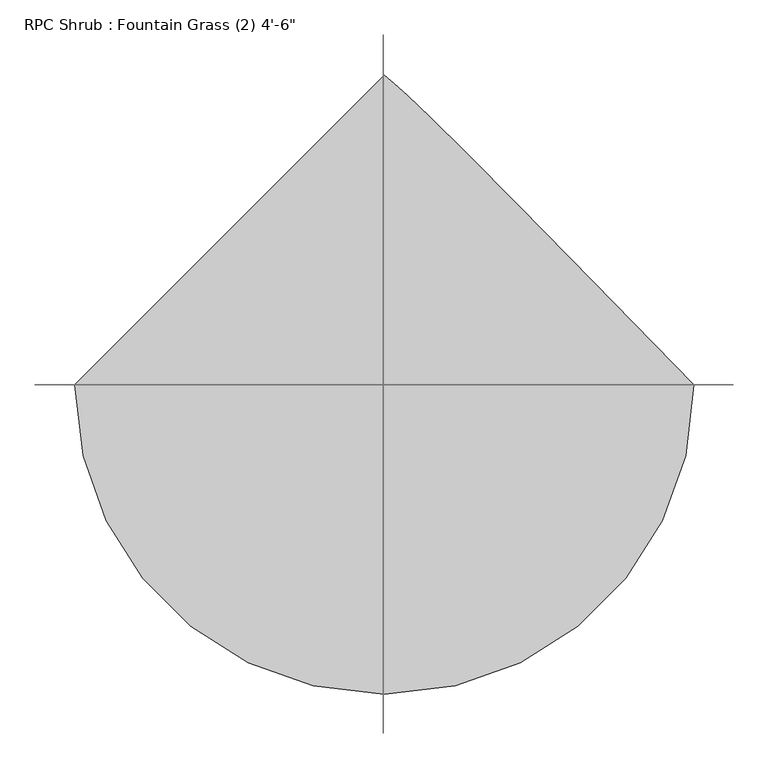
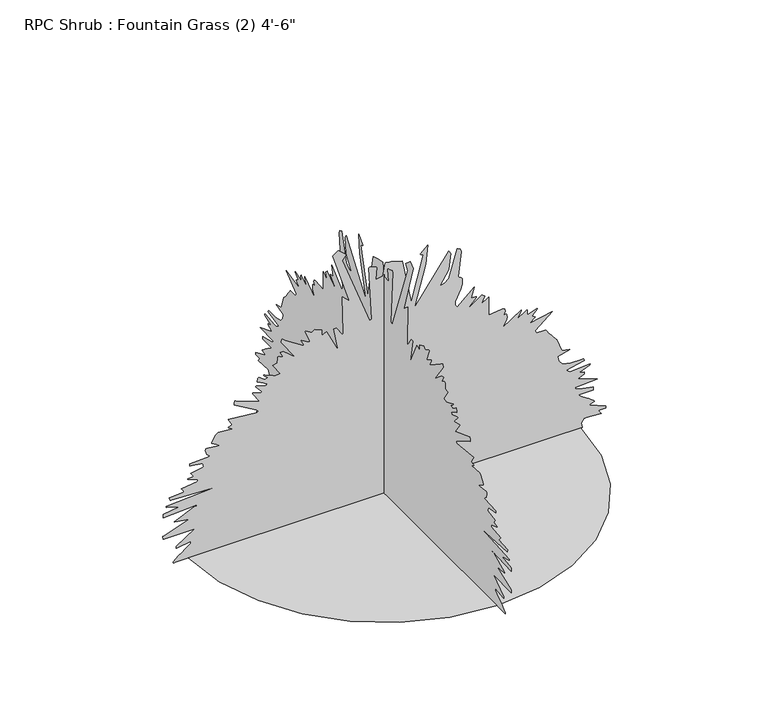
"""IFC4 building model written with IfcOpenShell, lengths in millimetres: geographic element geometry."""

from ifc_helpers import new_model, si_unit, origin, place, context, project, spatial, triangles, source, transform, mapped, element, save


def geographic_element_87ae7408(model_context):
    return source(origin(), model_context, "Body", "Tessellation", [
        triangles([(-987.0455658, 0.0, 0.0001807), (-960.952173, -226.1654466, 0.0001807), (-886.6343983, -433.862035, 0.0001807), (-770.0484913, -617.1406734, 0.0001807), (-617.1406734, -770.0484913, 0.0001807), (-433.862035, -886.6343983, 0.0001807), (-226.1654466, -960.952173, 0.0001807), (4.31e-05, -987.0455658, 0.0001807), (226.1657009, -960.952173, 0.0001807), (433.862035, -886.6343983, 0.0001807), (617.1406734, -770.0484913, 0.0001807), (770.0484913, -617.1406734, 0.0001807), (886.6343983, -433.862035, 0.0001807), (960.952173, -226.1654466, 0.0001807), (987.0455658, 8.63e-05, 0.0001807), (666.2769184, 329.0287173, 0.0001807), (428.4772619, 571.2784656, 0.0001807), (259.8137924, 741.2118793, 0.0001807), (146.4631077, 853.2918114, 0.0001807), (74.5956602, 921.9810053, 0.0001807), (30.3837036, 961.7446392, 0.0001807), (-0.0001294, 987.0455658, 0.0001807), (-192.732222, -8.8e-06, 1335.7745705), (-213.2038286, -7.2e-06, 1310.1839813), (-75.0206025, 1.47e-05, 941.6939009), (-74.0421966, 1.47e-05, 941.9784039), (-72.5994794, 1.47e-05, 942.7098999), (-70.8743122, 1.46e-05, 943.7080948), (-69.0480519, 1.45e-05, 944.7977812), (-67.3038361, 1.45e-05, 945.7985195), (-65.8220043, 1.44e-05, 946.5300882), (-64.7846675, 1.44e-05, 946.8119751), (-80.1384406, -2.1e-06, 1223.1789722), (-79.3512975, -2.1e-06, 1223.3695129), (-78.4244554, -2.1e-06, 1223.8850338), (-77.4526488, -2.1e-06, 1224.6394936), (-76.5311389, -2.2e-06, 1225.5436535), (-75.2199908, -2.3e-06, 1227.4587982), (-75.0206025, -2.4e-06, 1228.2971191), (-39.1952093, -1.4e-06, 1212.9427511), (-44.3130519, 2.2e-06, 1151.5281858), (-8.4877319, 1.9e-06, 1156.6462601), (4.7327266, -1.8e-06, 1221.0427654), (6.8660195, -2.1e-06, 1223.1789722), (43.5436857, -1.6e-06, 1215.9958351), (88.7523407, -8e-07, 1202.7066027), (134.8136643, 1.32e-05, 967.2843447), (196.2285203, -5e-07, 1197.5909992), (183.550624, -1e-06, 1203.2526449), (181.3428736, -1.1e-06, 1205.4269308), (180.8747518, -1.1e-06, 1207.8246769), (216.700145, -3.3e-06, 1243.6512691), (206.4644507, 2.5e-06, 1146.4100389), (150.1674419, 1.53e-05, 931.4576797), (324.1773419, -3.2e-06, 1172.2011972), (334.4109833, -2.3e-06, 1156.8469019), (324.1773419, 2.6e-06, 1074.959967), (278.1144741, 6.8e-06, 1003.3091806), (303.186799, 6.4e-06, 1010.2737991), (322.3333048, 5.3e-06, 1028.8183794), (365.1195376, -3.2e-06, 1172.2011972), (380.7405318, -2.8e-06, 1165.3635332), (386.8136713, -1.8e-06, 1149.1050053), (371.0377447, 5.8e-06, 1020.4236883), (372.5033166, 6e-06, 1017.0835579), (375.3150999, 6.2e-06, 1014.6375589), (378.9295232, 6.3e-06, 1012.7299719), (382.8157322, 6.4e-06, 1011.0028244), (386.4301191, 6.5e-06, 1009.0952374), (389.2419024, 6.6e-06, 1006.6492384), (390.7100178, 6.8e-06, 1003.3091806), (390.8116467, 8.5e-06, 974.9780611), (383.7479064, 1e-05, 950.4898756), (355.0433722, 1.34e-05, 892.7557543), (354.7944775, 1.44e-05, 876.299128), (365.1195376, 1.54e-05, 860.0101513), (452.1246194, 1.08e-05, 936.7764685), (436.7703604, 1.39e-05, 885.5980516), (437.4358357, 1.38e-05, 884.2035873), (460.8495229, 1.41e-05, 882.1284233), (462.3608042, 1.42e-05, 880.4799774), (460.8800079, 1.46e-05, 876.8274387), (425.4318083, 1.61e-05, 841.6561117), (426.5341393, 1.66e-05, 839.537709), (430.7911832, 1.6e-05, 840.3353348), (487.9487409, 1.42e-05, 880.4799774), (489.1120783, 1.43e-05, 881.361319), (491.0831062, 1.43e-05, 880.6425402), (503.3030362, 1.48e-05, 870.2437563), (487.9487409, 1.69e-05, 834.4196348), (523.7754058, 1.54e-05, 860.0101513), (523.7754058, 2.12e-05, 762.7688484), (593.7116893, 2.08e-05, 769.8782982), (604.2222033, 2.1e-05, 765.8219324), (607.2778307, 2.16e-05, 755.5679798), (600.5443027, 2.27e-05, 737.1784046), (610.7779804, 2.27e-05, 737.1784046), (611.8422323, 2.27e-05, 736.5230667), (614.1129513, 2.29e-05, 734.0897123), (616.2186367, 2.32e-05, 729.1722799), (616.7773962, 2.37e-05, 721.0722656), (614.4152584, 2.44e-05, 709.086006), (595.4261922, 2.67e-05, 670.6456924), (687.546841, 2.3e-05, 732.0602577), (687.8186268, 2.35e-05, 728.1842588), (667.0770149, 2.55e-05, 691.118062), (716.0887762, 2.38e-05, 722.0933516), (718.2554317, 2.36e-05, 721.8266527), (719.3450455, 2.39e-05, 719.0986942), (717.5061316, 2.5e-05, 697.6534916), (718.2554317, 2.51e-05, 696.2361362), (720.4347319, 2.49e-05, 695.6976517), (766.5382404, 2.45e-05, 712.7029364), (769.4337759, 2.42e-05, 711.5904316), (768.6387663, 2.44e-05, 709.4415802), (744.2522461, 2.59e-05, 683.2440514), (743.8433321, 2.61e-05, 680.8819136), (759.1976274, 2.67e-05, 670.6456924), (728.4915802, 2.82e-05, 645.0577194), (845.0825741, 2.67e-05, 669.6881201), (759.1976274, 3.09e-05, 598.994906), (764.3157017, 3.19e-05, 583.6431541), (810.3760443, 3.19e-05, 583.6431541), (812.6900019, 3.21e-05, 579.4623047), (818.8519804, 3.26e-05, 570.8923699), (827.7013676, 3.33e-05, 559.353176), (838.0696301, 3.41e-05, 546.269636), (848.7985537, 3.49e-05, 533.064192), (858.7223665, 3.56e-05, 521.1643006), (866.6750788, 3.61e-05, 511.9923677), (892.2629791, 4.01e-05, 445.4596919), (933.2077909, 4.07e-05, 435.2234708), (871.793153, 4.16e-05, 419.8692118), (876.9112272, 4.31e-05, 394.2787316), (879.8754358, 4.33e-05, 391.6269676), (882.8904408, 4.35e-05, 388.2919604), (885.7733316, 4.37e-05, 384.6267408), (888.3361839, 4.39e-05, 380.9920063), (890.3960873, 4.41e-05, 377.7407876), (891.7651897, 4.43e-05, 375.2261882), (892.2629791, 4.44e-05, 373.8088692), (895.890156, 4.44e-05, 372.7801892), (938.3258652, 4.5e-05, 363.5726844), (999.7404305, 4.5e-05, 363.5726844), (1000.5278824, 4.5e-05, 362.5440044), (1001.4549334, 4.51e-05, 361.080976), (1002.425223, 4.52e-05, 359.3588428), (1003.3472597, 4.53e-05, 357.5503776), (1004.1219217, 4.54e-05, 355.8282443), (1004.6578629, 4.55e-05, 354.3652159), (1004.8585773, 4.56e-05, 353.3364996), (912.7354214, 4.68e-05, 332.86413), (913.6015022, 4.69e-05, 331.6373154), (915.8976557, 4.7e-05, 329.6383458), (919.1819029, 4.71e-05, 327.1415142), (923.0020912, 4.73e-05, 324.4110123), (926.9110823, 4.75e-05, 321.7160823), (930.4620283, 4.76e-05, 319.3259302), (933.2077909, 4.77e-05, 317.5123781), (949.6695042, 4.77e-05, 318.6757155), (1032.0797356, 4.76e-05, 324.6954789), (1035.5645519, 4.74e-05, 322.6279452), (1033.032221, 4.76e-05, 319.7526484), (979.2680609, 4.89e-05, 297.0400085), (1004.8585773, 4.92e-05, 291.9219162), (1004.8585773, 4.99e-05, 281.6857132), (975.3971489, 5.07e-05, 267.6446189), (974.1499866, 5.08e-05, 266.331436), (1071.3912169, 5.29e-05, 230.5068058), (958.7956913, 5.32e-05, 225.3889678), (958.7956913, 5.35e-05, 220.2708572), (979.2680609, 5.41e-05, 210.0351811), (1050.9188473, 5.5e-05, 194.6814126), (1050.9188473, 5.6e-05, 179.327626), (974.1499866, 5.6e-05, 179.327626), (978.767728, 5.62e-05, 175.5818881), (990.6523224, 5.67e-05, 167.0838239), (1006.8625975, 5.74e-05, 155.6789786), (1024.4520761, 5.81e-05, 143.2134423), (1051.9830992, 5.94e-05, 122.4842661), (1056.0369942, 5.96e-05, 117.9127791), (1055.1428627, 5.97e-05, 116.2480642), (1031.9527084, 6.02e-05, 108.5996212), (1030.4464777, 6.02e-05, 107.6770939), (1112.3334852, 6.24e-05, 71.8517007), (1112.3334852, 6.3e-05, 61.6157658), (1076.5093637, 6.3e-05, 61.6157658), (1088.8461107, 6.4e-05, 43.7974311), (1091.8611156, 6.42e-05, 41.1441501), (1004.8585773, 6.39e-05, 46.2622425), (989.504282, 6.51e-05, 25.7906269), (994.6223562, 6.66e-05, 0.2009925), (-1062.775609, 7.09e-05, 6.89e-05), (-1062.775609, 7.05e-05, 5.1179681), (-1049.4888474, 6.99e-05, 15.7529118), (-1033.944084, 6.92e-05, 27.9602914), (-1017.6728388, 6.84e-05, 40.5703616), (-1002.191589, 6.77e-05, 52.4138656), (-989.0343979, 6.71e-05, 62.3213777), (-979.7176701, 6.67e-05, 69.1234924), (-975.7730707, 6.66e-05, 71.6507864), (-975.7730707, 6.6e-05, 81.8864716), (-1047.4213137, 6.66e-05, 71.6507864), (-1047.4213137, 6.6e-05, 81.8864716), (-955.3006285, 6.23e-05, 143.3013185), (-1113.9564966, 6.23e-05, 143.3013185), (-1114.0479881, 6.22e-05, 144.6553964), (-1114.2638906, 6.21e-05, 147.0447673), (-1114.5102419, 6.19e-05, 150.0158069), (-1114.6931522, 6.17e-05, 153.1156177), (-1114.7261444, 6.16e-05, 155.891066), (-1114.5102419, 6.14e-05, 157.8885276), (-1113.9564966, 6.14e-05, 158.6551051), (-986.0066757, 5.87e-05, 204.7161744), (-1054.7643974, 5.81e-05, 213.3275311), (-1057.6574621, 5.8e-05, 214.9521049), (-955.3006285, 5.53e-05, 261.0126836), (-945.06448, 5.53e-05, 261.0126836), (-945.06448, 5.5e-05, 266.130776), (-1113.9564966, 5.56e-05, 255.8945912), (-1113.9564966, 5.44e-05, 276.3669608), (-1032.0695618, 5.38e-05, 286.6031456), (-1098.6022739, 5.26e-05, 307.0755152), (-1098.6022739, 5.22e-05, 312.1910823), (-852.941324, 5.13e-05, 327.5453776), (-1078.1298317, 5.07e-05, 337.7815624), (-1082.9660191, 4.99e-05, 351.3121319), (-1083.2479786, 4.98e-05, 353.1358578), (-1006.4790453, 4.95e-05, 358.253932), (-1021.1679016, 4.84e-05, 377.3064754), (-1021.8333406, 4.83e-05, 378.7237945), (-939.9464058, 4.77e-05, 388.9599792), (-939.9464058, 4.71e-05, 399.196164), (-983.6648129, 4.62e-05, 414.4208888), (-989.0952953, 4.6e-05, 417.5603411), (-991.1248226, 4.58e-05, 419.6685336), (-960.4187754, 4.55e-05, 424.7866442), (-975.1050156, 4.44e-05, 443.8391513), (-975.7730707, 4.43e-05, 445.2590137), (-909.2403585, 4.37e-05, 455.4926551), (-914.3558893, 4.25e-05, 475.965061), (-980.8911449, 4.19e-05, 486.2012458), (-980.8911449, 4.13e-05, 496.4374306), (-878.5317678, 4.1e-05, 501.5555048), (-879.1134184, 4.09e-05, 503.3716003), (-888.6028828, 4.02e-05, 513.6840159), (-893.8860632, 4e-05, 516.9098001), (-900.7211838, 3.88e-05, 540.5851356), (-900.558621, 3.85e-05, 544.4840255), (-899.0041374, 3.82e-05, 547.6158474), (-894.7090508, 3.84e-05, 548.9721963), (-839.7257063, 3.85e-05, 543.0539892), (-832.4714979, 3.85e-05, 542.4977368), (-834.0945093, 3.85e-05, 545.8555987), (-865.9461262, 3.72e-05, 565.5888419), (-868.2956194, 3.7e-05, 568.088217), (-868.4048424, 3.65e-05, 572.164894), (-848.5039495, 3.46e-05, 604.96896), (-842.4562082, 3.44e-05, 611.1792641), (-837.5895721, 3.42e-05, 614.1485596), (-765.9387857, 3.46e-05, 609.030449), (-780.5183464, 3.41e-05, 617.4352776), (-785.6364206, 3.37e-05, 622.5609821), (-786.4086119, 3.36e-05, 624.384708), (-767.3586119, 3.34e-05, 628.6646067), (-765.9387857, 3.33e-05, 629.5027822), (-786.4086119, 3.12e-05, 665.3269037), (-637.9889648, 3.21e-05, 649.9752245), (-637.7984241, 3.21e-05, 650.9530718), (-637.2828306, 3.2e-05, 652.395789), (-636.5284435, 3.19e-05, 654.1204657), (-635.6242109, 3.18e-05, 655.946735), (-634.6564648, 3.17e-05, 657.6916866), (-633.7090662, 3.16e-05, 659.1725555), (-632.8733614, 3.15e-05, 660.2088295), (-755.7025646, 2.72e-05, 731.8596159), (-755.710195, 2.71e-05, 734.6180958), (-755.6593987, 2.69e-05, 738.1944036), (-755.4384092, 2.67e-05, 742.1339161), (-754.9329895, 2.65e-05, 745.9743793), (-754.0313004, 2.63e-05, 749.26117), (-752.6190319, 2.61e-05, 751.5344324), (-750.5844904, 2.6e-05, 752.3319855), (-627.7552872, 2.88e-05, 706.2717155), (-663.6860882, 2.56e-05, 759.6675116), (-663.5794086, 2.54e-05, 762.5682066), (-660.4755283, 2.56e-05, 763.5054314), (-620.4934484, 2.58e-05, 751.3083561), (-617.5191387, 2.6e-05, 752.3319855), (-618.27854, 2.56e-05, 755.4434961), (-647.6638103, 2.37e-05, 790.1982788), (-648.2251133, 2.36e-05, 793.2742538), (-645.0653498, 2.38e-05, 794.1149729), (-597.0467328, 2.45e-05, 777.9225019), (-596.4675894, 2.44e-05, 778.9130665), (-595.0452198, 2.43e-05, 780.3888485), (-593.2570295, 2.42e-05, 782.1490608), (-591.5755551, 2.41e-05, 784.0032354), (-590.4782747, 2.4e-05, 785.7507305), (-590.4376522, 2.39e-05, 787.201078), (-591.9286222, 2.39e-05, 788.1586504), (-637.9889648, 2.24e-05, 813.7466234), (-639.6145197, 2.21e-05, 815.2045286), (-640.0666723, 2.19e-05, 818.265243), (-638.3851616, 2.15e-05, 826.5253492), (-636.7163681, 2.14e-05, 830.3861601), (-634.8012234, 2.12e-05, 833.1724726), (-632.8733614, 2.11e-05, 834.218993), (-630.4730719, 2.12e-05, 834.2443548), (-602.164807, 2.24e-05, 813.7466234), (-586.810548, 2.2e-05, 818.8646976), (-606.0256179, 2.11e-05, 834.9200403), (-607.7909171, 2.1e-05, 837.6987951), (-607.2829176, 2.08e-05, 839.3370672), (-603.6684943, 2.09e-05, 838.9128925), (-561.8702826, 2.2e-05, 820.0915123), (-550.9864265, 2.24e-05, 813.7466234), (-525.3959464, 2.2e-05, 818.8646976), (-559.8662261, 1.89e-05, 871.7906096), (-561.2226113, 1.87e-05, 875.1611887), (-540.7502054, 1.84e-05, 880.2793356), (-537.9714506, 1.73e-05, 906.7536644), (-536.9859366, 1.7e-05, 909.870262), (-535.6321312, 1.66e-05, 910.9878536), (-533.2191244, 1.68e-05, 912.2654646), (-529.3558064, 1.69e-05, 911.5212513), (-510.0416511, 1.72e-05, 900.7517052), (-525.3959464, 1.53e-05, 931.4576797), (-510.0416511, 1.53e-05, 931.4576797), (-448.6270494, 1.84e-05, 880.2793356), (-520.2778358, 1.23e-05, 982.63864), (-520.4962818, 1.22e-05, 984.7163475), (-516.051277, 1.16e-05, 996.9642191), (-515.2257823, 1.15e-05, 998.3459661), (-515.1597616, 1.14e-05, 997.9903919), (-498.3728866, 1.21e-05, 985.7882298), (-408.0734565, 1.55e-05, 927.9093498), (-402.5667432, 1.56e-05, 926.342149), (-417.4790597, 1.45e-05, 951.9148613), (-418.5687098, 1.42e-05, 955.282897), (-417.9210385, 1.38e-05, 957.0481962), (-415.5080317, 1.41e-05, 957.1853245), (-380.6389392, 1.48e-05, 937.1701944), (-376.976263, 1.5e-05, 936.5758266), (-376.9203798, 1.43e-05, 940.7439589), (-397.9032924, 1.21e-05, 994.048336), (-397.4486326, 1.14e-05, 997.9903919), (-395.0686543, 1.16e-05, 998.5085289), (-366.1584277, 1.23e-05, 982.382115), (-351.3883264, 1.17e-05, 992.8748611), (-315.5616614, 1.26e-05, 977.5205658), (-315.5616614, 1.44e-05, 946.8119751), (-294.1621864, 1.4e-05, 958.3587994), (-291.1294318, 1.39e-05, 958.6407589), (-289.9737247, 1.38e-05, 957.0481962), (-233.6754533, 2.08e-05, 839.3370672), (-254.1470598, 1.35e-05, 962.1662704), (-243.9113837, 1.35e-05, 962.1662704), (-213.2038286, 1.62e-05, 916.1059278), (-211.0877513, 1.6e-05, 916.598703), (-209.5368286, 1.59e-05, 917.6680418), (-208.4642015, 1.57e-05, 919.1971636), (-207.7817031, 1.56e-05, 921.0716858), (-207.4032379, 1.54e-05, 923.1722116), (-207.2399121, 1.53e-05, 925.3845766), (-207.2046126, 1.52e-05, 927.5918547), (-213.2038286, 4.4e-06, 1115.7040644), (-210.5383663, 4.8e-06, 1115.4424524), (-179.2496511, 6.1e-06, 1087.4745375), (-177.3786897, 6.2e-06, 1084.9954737), (-259.2651522, -9.7e-06, 1351.1262497), (-233.6754533, -1.09e-05, 1371.5986919), (-3.3699163, -189.3624059, 1335.7745705), (-3.3699163, -209.8340125, 1310.1839813), (-3.3699163, -71.6505366, 941.6939009), (-3.3699163, -70.6721261, 941.9784039), (-3.3699163, -69.2296633, 942.7098999), (-3.3699163, -67.5042417, 943.7080948), (-3.3699163, -65.6782403, 944.7977812), (-3.3699163, -63.93402, 945.7985195), (-3.3699163, -62.4519338, 946.5300882), (-3.3699163, -61.4148514, 946.8119751), (-3.3699163, -76.7683792, 1223.1789722), (-3.3699163, -75.9812316, 1223.3695129), (-3.3699163, -75.054385, 1223.8850338), (-3.3699163, -74.0828373, 1224.6394936), (-3.3699163, -73.161073, 1225.5436535), (-3.3699163, -71.8499249, 1227.4587982), (-3.3699163, -71.6505366, 1228.2971191), (-3.3699163, -35.8251411, 1212.9427511), (-3.3699163, -40.9429814, 1151.5281858), (-3.3699163, -5.1177648, 1156.6462601), (-3.3699163, 8.1026934, 1221.0427654), (-3.3699163, 10.2359611, 1223.1789722), (-3.3699163, 46.9137516, 1215.9958351), (-3.3699163, 92.122402, 1202.7066027), (-3.3699163, 138.1834804, 967.2843447), (-3.3699163, 199.5985907, 1197.5909992), (-3.3699163, 186.9206945, 1203.2526449), (-3.3699163, 184.7129259, 1205.4269308), (-3.3699163, 184.244804, 1207.8246769), (-3.3699163, 220.0701972, 1243.6512691), (-3.3699163, 209.8342668, 1146.4100389), (-3.3699163, 153.5372671, 931.4576797), (-3.3699163, 327.5453776, 1172.2011972), (-3.3699163, 337.7815624, 1156.8469019), (-3.3699163, 327.5453776, 1074.959967), (-3.3699163, 281.4850532, 1003.3091806), (-3.3699163, 306.5573782, 1010.2737991), (-3.3699163, 325.7038839, 1028.8183794), (-3.3699163, 368.4901168, 1172.2011972), (-3.3699163, 384.1085675, 1165.3635332), (-3.3699163, 390.1842505, 1149.1050053), (-3.3699163, 374.4057804, 1020.4236883), (-3.3699163, 375.8738957, 1017.0835579), (-3.3699163, 378.6856791, 1014.6375589), (-3.3699163, 382.3001023, 1012.7299719), (-3.3699163, 386.1863113, 1011.0028244), (-3.3699163, 389.8006983, 1009.0952374), (-3.3699163, 392.6124816, 1006.6492384), (-3.3699163, 394.0780535, 1003.3091806), (-3.3699163, 394.1796824, 974.9780611), (-3.3699163, 387.1184855, 950.4898756), (-3.3699163, 358.4139513, 892.7557543), (-3.3699163, 358.1650566, 876.299128), (-3.3699163, 368.4901168, 860.0101513), (-3.3699163, 455.4926551, 936.7764685), (-3.3699163, 440.1409032, 885.5980516), (-3.3699163, 440.8038714, 884.2035873), (-3.3699163, 464.2175586, 882.1284233), (-3.3699163, 465.7288399, 880.4799774), (-3.3699163, 464.2505871, 876.8274387), (-3.3699163, 428.8023874, 841.6561117), (-3.3699163, 429.9047184, 839.537709), (-3.3699163, 434.1617623, 840.3353348), (-3.3699163, 491.31932, 880.4799774), (-3.3699163, 492.480114, 881.361319), (-3.3699163, 494.4536854, 880.6425402), (-3.3699163, 506.6736154, 870.2437563), (-3.3699163, 491.31932, 834.4196348), (-3.3699163, 527.1434415, 860.0101513), (-3.3699163, 527.1434415, 762.7688484), (-3.3699163, 597.079725, 769.8782982), (-3.3699163, 607.5927824, 765.8219324), (-3.3699163, 610.6458664, 755.5679798), (-3.3699163, 603.9123384, 737.1784046), (-3.3699163, 614.1485596, 737.1784046), (-3.3699163, 615.2128115, 736.5230667), (-3.3699163, 617.4835304, 734.0897123), (-3.3699163, 619.5866724, 729.1722799), (-3.3699163, 620.1479753, 721.0722656), (-3.3699163, 617.7858376, 709.086006), (-3.3699163, 598.7942279, 670.6456924), (-3.3699163, 690.9174202, 732.0602577), (-3.3699163, 691.1866625, 728.1842588), (-3.3699163, 670.4450506, 691.118062), (-3.3699163, 719.4568119, 722.0933516), (-3.3699163, 721.6260109, 721.8266527), (-3.3699163, 722.7156246, 719.0986942), (-3.3699163, 720.8767107, 697.6534916), (-3.3699163, 721.6260109, 696.2361362), (-3.3699163, 723.805311, 695.6976517), (-3.3699163, 769.9062761, 712.7029364), (-3.3699163, 772.804355, 711.5904316), (-3.3699163, 772.0093454, 709.4415802), (-3.3699163, 747.6202818, 683.2440514), (-3.3699163, 747.2139112, 680.8819136), (-3.3699163, 762.5682066, 670.6456924), (-3.3699163, 731.8596159, 645.0577194), (-3.3699163, 848.4531532, 669.6881201), (-3.3699163, 762.5682066, 598.994906), (-3.3699163, 767.6862808, 583.6431541), (-3.3699163, 813.7466234, 583.6431541), (-3.3699163, 816.0605083, 579.4623047), (-3.3699163, 822.2225595, 570.8923699), (-3.3699163, 831.0694033, 559.353176), (-3.3699163, 841.4402092, 546.269636), (-3.3699163, 852.1691328, 533.064192), (-3.3699163, 862.0904022, 521.1643006), (-3.3699163, 870.0431145, 511.9923677), (-3.3699163, 895.6335583, 445.4596919), (-3.3699163, 936.5758266, 435.2234708), (-3.3699163, 875.1611887, 419.8692118), (-3.3699163, 880.2793356, 394.2787316), (-3.3699163, 883.246015, 391.6269676), (-3.3699163, 886.2610199, 388.289417), (-3.3699163, 889.1439108, 384.6267408), (-3.3699163, 891.7067631, 380.9920063), (-3.3699163, 893.764123, 377.7407876), (-3.3699163, 895.1357689, 375.2261882), (-3.3699163, 895.6335583, 373.8088692), (-3.3699163, 899.2607351, 372.7801892), (-3.3699163, 941.6939009, 363.5726844), (-3.3699163, 1003.1084661, 363.5726844), (-3.3699163, 1003.8959181, 362.5440044), (-3.3699163, 1004.8229691, 361.080976), (-3.3699163, 1005.7958021, 359.3588428), (-3.3699163, 1006.7178389, 357.5503776), (-3.3699163, 1007.4925009, 355.8282443), (-3.3699163, 1008.028442, 354.3652159), (-3.3699163, 1008.226613, 353.3364996), (-3.3699163, 916.1059278, 332.86413), (-3.3699163, 916.9695379, 331.6373154), (-3.3699163, 919.2682348, 329.6383458), (-3.3699163, 922.5499386, 327.1415142), (-3.3699163, 926.3701269, 324.4110123), (-3.3699163, 930.279118, 321.7160823), (-3.3699163, 933.8326075, 319.3259302), (-3.3699163, 936.5758266, 317.5098347), (-3.3699163, 953.0400833, 318.6757155), (-3.3699163, 1035.4503147, 324.6954789), (-3.3699163, 1038.9351311, 322.6279452), (-3.3699163, 1036.4028002, 319.7501049), (-3.3699163, 982.63864, 297.0400085), (-3.3699163, 1008.226613, 291.9219162), (-3.3699163, 1008.226613, 281.6857132), (-3.3699163, 978.767728, 267.6446189), (-3.3699163, 977.5205658, 266.331436), (-3.3699163, 1074.7592525, 230.5068058), (-3.3699163, 962.1662704, 225.3887135), (-3.3699163, 962.1662704, 220.2708572), (-3.3699163, 982.63864, 210.0351811), (-3.3699163, 1054.2894264, 194.6814126), (-3.3699163, 1054.2894264, 179.327626), (-3.3699163, 977.5205658, 179.327626), (-3.3699163, 982.1357637, 175.5818881), (-3.3699163, 994.0229015, 167.0835696), (-3.3699163, 1010.2331766, 155.6787243), (-3.3699163, 1027.8226553, 143.2131879), (-3.3699163, 1055.3536783, 122.4842661), (-3.3699163, 1059.4075733, 117.9127791), (-3.3699163, 1058.5134418, 116.2478099), (-3.3699163, 1035.3207441, 108.5993669), (-3.3699163, 1033.8170568, 107.6768396), (-3.3699163, 1115.7040644, 71.8517007), (-3.3699163, 1115.7040644, 61.6157658), (-3.3699163, 1079.8773994, 61.6157658), (-3.3699163, 1092.2166899, 43.7971768), (-3.3699163, 1095.2316948, 41.1441501), (-3.3699163, 1008.226613, 46.2619882), (-3.3699163, 992.8748611, 25.7903726), (-3.3699163, 997.9929354, 0.2009237), (-3.3699163, -1059.4050299, 0.0), (-3.3699163, -1059.4050299, 5.117917), (-3.3699163, -1046.1182682, 15.7528607), (-3.3699163, -1030.5760483, 27.9600371), (-3.3699163, -1014.3022596, 40.5701072), (-3.3699163, -998.8235533, 52.4138656), (-3.3699163, -985.6638187, 62.3213777), (-3.3699163, -976.3496344, 69.1234924), (-3.3699163, -972.4024916, 71.6507864), (-3.3699163, -972.4024916, 81.8864716), (-3.3699163, -1044.053278, 71.6507864), (-3.3699163, -1044.053278, 81.8864716), (-3.3699163, -951.930122, 143.3013185), (-3.3699163, -1110.5859175, 143.3013185), (-3.3699163, -1110.677409, 144.6553964), (-3.3699163, -1110.8933115, 147.0447673), (-3.3699163, -1111.1396627, 150.0158069), (-3.3699163, -1111.3251165, 153.1156177), (-3.3699163, -1111.3555653, 155.891066), (-3.3699163, -1111.1396627, 157.8885276), (-3.3699163, -1110.5859175, 158.6551051), (-3.3699163, -982.63864, 204.7161744), (-3.3699163, -1051.3938183, 213.3275311), (-3.3699163, -1054.2894264, 214.9521049), (-3.3699163, -951.930122, 261.0126836), (-3.3699163, -941.6939009, 261.0126836), (-3.3699163, -941.6939009, 266.130776), (-3.3699163, -1110.5859175, 255.8945912), (-3.3699163, -1110.5859175, 276.3669608), (-3.3699163, -1028.6989826, 286.6031456), (-3.3699163, -1095.2316948, 307.0755152), (-3.3699163, -1095.2316948, 312.1910823), (-3.3699163, -849.5732883, 327.5453776), (-3.3699163, -1074.7592525, 337.7815624), (-3.3699163, -1079.5954399, 351.3121319), (-3.3699163, -1079.8773994, 353.1358578), (-3.3699163, -1003.1084661, 358.253932), (-3.3699163, -1017.7973225, 377.3064754), (-3.3699163, -1018.4627615, 378.7237945), (-3.3699163, -936.5758266, 388.9599792), (-3.3699163, -936.5758266, 399.196164), (-3.3699163, -980.2942337, 414.4208888), (-3.3699163, -985.7272596, 417.5603411), (-3.3699163, -987.7567869, 419.6685336), (-3.3699163, -957.0481962, 424.7866442), (-3.3699163, -971.7369799, 443.8391513), (-3.3699163, -972.4024916, 445.2590137), (-3.3699163, -905.8697794, 455.4926551), (-3.3699163, -910.9878536, 475.965061), (-3.3699163, -977.5205658, 486.2012458), (-3.3699163, -977.5205658, 496.4374306), (-3.3699163, -875.1611887, 501.5555048), (-3.3699163, -875.7428392, 503.3690932), (-3.3699163, -885.2348471, 513.6814725), (-3.3699163, -890.515484, 516.9098001), (-3.3699163, -897.3506046, 540.5851356), (-3.3699163, -897.1880419, 544.4840255), (-3.3699163, -895.6335583, 547.6158474), (-3.3699163, -891.3384716, 548.9721963), (-3.3699163, -836.3576706, 543.0539892), (-3.3699163, -829.1009188, 542.4977368), (-3.3699163, -830.7239302, 545.8555987), (-3.3699163, -862.5780905, 565.5888419), (-3.3699163, -864.9250402, 568.088217), (-3.3699163, -865.0368067, 572.1623506), (-3.3699163, -845.1333704, 604.96896), (-3.3699163, -839.0856291, 611.1792641), (-3.3699163, -834.218993, 614.1485596), (-3.3699163, -762.5682066, 609.030449), (-3.3699163, -777.1477673, 617.4352776), (-3.3699163, -782.2658415, 622.5609821), (-3.3699163, -783.0405762, 624.384708), (-3.3699163, -763.9880327, 628.6646067), (-3.3699163, -762.5682066, 629.5027822), (-3.3699163, -783.0405762, 665.3269037), (-3.3699163, -634.6209291, 649.9752245), (-3.3699163, -634.427845, 650.9530718), (-3.3699163, -633.9122515, 652.395789), (-3.3699163, -633.1604078, 654.1204657), (-3.3699163, -632.2561752, 655.946735), (-3.3699163, -631.2858856, 657.6916866), (-3.3699163, -630.3410305, 659.1725555), (-3.3699163, -629.5027822, 660.2088295), (-3.3699163, -752.3319855, 731.8596159), (-3.3699163, -752.3396158, 734.6180958), (-3.3699163, -752.291363, 738.1944036), (-3.3699163, -752.0703735, 742.1339161), (-3.3699163, -751.5649538, 745.9743793), (-3.3699163, -750.6632647, 749.26117), (-3.3699163, -749.2484528, 751.5344324), (-3.3699163, -747.2139112, 752.3319855), (-3.3699163, -624.384708, 706.2717155), (-3.3699163, -660.315509, 759.6675116), (-3.3699163, -660.2088295, 762.5682066), (-3.3699163, -657.1049492, 763.5054314), (-3.3699163, -617.1228693, 751.3083561), (-3.3699163, -614.1485596, 752.3319855), (-3.3699163, -614.9079609, 755.4434961), (-3.3699163, -644.2932312, 790.1982788), (-3.3699163, -644.8570776, 793.2742538), (-3.3699163, -641.6947706, 794.1149729), (-3.3699163, -593.6761537, 777.9225019), (-3.3699163, -593.0970102, 778.9130665), (-3.3699163, -591.6771841, 780.3888485), (-3.3699163, -589.8864867, 782.1490608), (-3.3699163, -588.2075194, 784.0032354), (-3.3699163, -587.1076956, 785.7507305), (-3.3699163, -587.0670731, 787.201078), (-3.3699163, -588.5580431, 788.1586504), (-3.3699163, -634.6209291, 813.7466234), (-3.3699163, -636.2439405, 815.2045286), (-3.3699163, -636.6960932, 818.265243), (-3.3699163, -635.0171259, 826.5253492), (-3.3699163, -633.3458616, 830.3861601), (-3.3699163, -631.4306442, 833.1724726), (-3.3699163, -629.5027822, 834.218993), (-3.3699163, -627.1050362, 834.2443548), (-3.3699163, -598.7942279, 813.7466234), (-3.3699163, -583.4399689, 818.8646976), (-3.3699163, -602.6575822, 834.9200403), (-3.3699163, -604.420338, 837.6987951), (-3.3699163, -603.9123384, 839.3370672), (-3.3699163, -600.2979152, 838.9128925), (-3.3699163, -558.5022469, 820.0915123), (-3.3699163, -547.6158474, 813.7466234), (-3.3699163, -522.0253673, 818.8646976), (-3.3699163, -556.495647, 871.7906096), (-3.3699163, -557.8520322, 875.1611887), (-3.3699163, -537.3796263, 880.2793356), (-3.3699163, -534.6008715, 906.7536644), (-3.3699163, -533.6153575, 909.870262), (-3.3699163, -532.261552, 910.9878536), (-3.3699163, -529.8510887, 912.2654646), (-3.3699163, -525.9877707, 911.5212513), (-3.3699163, -506.6736154, 900.7517052), (-3.3699163, -522.0253673, 931.4576797), (-3.3699163, -506.6736154, 931.4576797), (-3.3699163, -445.2564703, 880.2793356), (-3.3699163, -516.9072567, 982.63864), (-3.3699163, -517.1282461, 984.7163475), (-3.3699163, -512.6832413, 996.9642191), (-3.3699163, -511.8552032, 998.3459661), (-3.3699163, -511.7891825, 997.9929354), (-3.3699163, -495.0023074, 985.7882298), (-3.3699163, -404.7028773, 927.9093498), (-3.3699163, -399.196164, 926.342149), (-3.3699163, -414.111024, 951.9148613), (-3.3699163, -415.1981306, 955.282897), (-3.3699163, -414.5504594, 957.0481962), (-3.3699163, -412.1374526, 957.1853245), (-3.3699163, -377.2709035, 937.1701944), (-3.3699163, -373.6056839, 936.5758266), (-3.3699163, -373.5523441, 940.7439589), (-3.3699163, -394.5327132, 994.048336), (-3.3699163, -394.0780535, 997.9929354), (-3.3699163, -391.6980752, 998.5085289), (-3.3699163, -362.790392, 982.382115), (-3.3699163, -348.0177472, 992.8748611), (-3.3699163, -312.1910823, 977.5205658), (-3.3699163, -312.1910823, 946.8119751), (-3.3699163, -290.7916072, 958.3587994), (-3.3699163, -287.7613961, 958.6407589), (-3.3699163, -286.6031456, 957.0481962), (-3.3699163, -230.3056372, 839.3370672), (-3.3699163, -250.7772437, 962.1662704), (-3.3699163, -240.5415676, 962.1662704), (-3.3699163, -209.8340125, 916.1059278), (-3.3699163, -207.7176991, 916.598703), (-3.3699163, -206.1670306, 917.6680418), (-3.3699163, -205.094131, 919.1971636), (-3.3699163, -204.411887, 921.0716858), (-3.3699163, -204.0334218, 923.1722116), (-3.3699163, -203.8698416, 925.3845766), (-3.3699163, -203.8347965, 927.5918547), (-3.3699163, -209.8340125, 1115.7040644), (-3.3699163, -207.1682958, 1115.4424524), (-3.3699163, -175.879835, 1087.4745375), (-3.3699163, -174.0086193, 1084.9954737), (-3.3699163, -255.8945912, 1351.1262497), (-3.3699163, -230.3056372, 1371.5986919)], [[21, 22, 1], [20, 21, 1], [19, 20, 1], [18, 19, 1], [17, 18, 1], [17, 1, 2], [17, 2, 3], [17, 3, 4], [16, 17, 4], [16, 4, 5], [16, 5, 6], [16, 6, 7], [16, 7, 8], [16, 8, 9], [16, 9, 10], [16, 10, 11], [16, 11, 12], [15, 16, 12], [14, 15, 12], [13, 14, 12], [168, 169, 170], [119, 120, 121], [131, 132, 133], [76, 77, 78], [188, 189, 190], [333, 334, 335], [215, 216, 217], [266, 267, 268], [90, 91, 92], [235, 236, 237], [234, 235, 237], [214, 215, 217], [103, 104, 105], [103, 105, 106], [327, 328, 329], [233, 234, 237], [54, 55, 56], [54, 56, 57], [54, 57, 58], [230, 231, 232], [117, 118, 119], [238, 239, 240], [229, 230, 232], [60, 61, 62], [60, 62, 63], [191, 192, 193], [161, 162, 163], [38, 39, 40], [356, 357, 358], [356, 358, 359], [237, 238, 240], [202, 203, 204], [202, 204, 205], [187, 188, 190], [319, 320, 321], [366, 367, 368], [366, 368, 369], [366, 369, 370], [227, 228, 229], [219, 220, 221], [219, 221, 222], [191, 193, 194], [191, 194, 195], [191, 195, 196], [191, 196, 197], [191, 197, 198], [191, 198, 199], [191, 199, 200], [191, 200, 201], [185, 186, 187], [184, 185, 187], [184, 187, 190], [173, 174, 175], [172, 173, 175], [113, 114, 115], [191, 201, 202], [191, 202, 205], [226, 227, 229], [225, 226, 229], [225, 229, 232], [150, 151, 152], [149, 150, 152], [148, 149, 152], [147, 148, 152], [146, 147, 152], [145, 146, 152], [144, 145, 152], [143, 144, 152], [372, 23, 24], [371, 372, 24], [370, 371, 24], [370, 24, 25], [366, 370, 25], [242, 243, 244], [241, 242, 244], [223, 224, 225], [222, 223, 225], [219, 222, 225], [205, 206, 207], [291, 292, 293], [333, 335, 336], [205, 207, 208], [76, 78, 79], [205, 208, 209], [205, 209, 210], [205, 210, 211], [205, 211, 212], [205, 212, 213], [205, 213, 214], [332, 333, 336], [331, 332, 336], [330, 331, 336], [330, 336, 337], [365, 366, 25], [37, 38, 40], [60, 63, 64], [262, 263, 264], [32, 33, 34], [313, 314, 315], [312, 313, 315], [311, 312, 315], [364, 365, 25], [164, 165, 166], [160, 161, 163], [160, 163, 164], [318, 319, 321], [37, 40, 41], [36, 37, 41], [35, 36, 41], [34, 35, 41], [32, 34, 41], [32, 41, 42], [112, 113, 115], [112, 115, 116], [171, 172, 175], [363, 364, 25], [262, 264, 265], [261, 262, 265], [346, 347, 348], [346, 348, 349], [285, 286, 287], [290, 291, 293], [290, 293, 294], [180, 181, 182], [233, 237, 240], [350, 351, 352], [340, 341, 342], [339, 340, 342], [338, 339, 342], [338, 342, 343], [284, 285, 287], [284, 287, 288], [179, 180, 182], [179, 182, 183], [179, 183, 184], [330, 337, 338], [80, 81, 82], [79, 80, 82], [76, 79, 82], [76, 82, 83], [261, 265, 266], [261, 266, 268], [356, 359, 360], [214, 217, 218], [205, 214, 218], [191, 205, 218], [191, 218, 219], [191, 219, 225], [190, 191, 225], [184, 190, 225], [179, 184, 225], [178, 179, 225], [177, 178, 225], [176, 177, 225], [175, 176, 225], [171, 175, 225], [170, 171, 225], [168, 170, 225], [107, 108, 109], [106, 107, 109], [106, 109, 110], [362, 363, 25], [122, 123, 124], [142, 143, 152], [112, 116, 117], [112, 117, 119], [111, 112, 119], [130, 131, 133], [275, 276, 277], [275, 277, 278], [275, 278, 279], [275, 279, 280], [275, 280, 281], [275, 281, 282], [275, 282, 283], [275, 283, 284], [353, 354, 355], [349, 350, 352], [346, 349, 352], [345, 346, 352], [344, 345, 352], [86, 87, 88], [289, 290, 294], [60, 64, 65], [59, 60, 65], [50, 51, 52], [49, 50, 52], [48, 49, 52], [48, 52, 53], [47, 48, 53], [47, 53, 54], [284, 288, 289], [164, 166, 167], [160, 164, 167], [160, 167, 168], [159, 160, 168], [159, 168, 225], [158, 159, 225], [157, 158, 225], [156, 157, 225], [155, 156, 225], [154, 155, 225], [153, 154, 225], [152, 153, 225], [142, 152, 225], [141, 142, 225], [140, 141, 225], [139, 140, 225], [138, 139, 225], [137, 138, 225], [136, 137, 225], [135, 136, 225], [134, 135, 225], [133, 134, 225], [130, 133, 225], [129, 130, 225], [128, 129, 225], [127, 128, 225], [126, 127, 225], [125, 126, 225], [124, 125, 225], [122, 124, 225], [121, 122, 225], [119, 121, 225], [111, 119, 225], [110, 111, 225], [225, 232, 233], [225, 233, 240], [43, 44, 45], [93, 94, 95], [93, 95, 96], [92, 93, 96], [311, 315, 316], [42, 43, 45], [42, 45, 46], [32, 42, 46], [32, 46, 47], [32, 47, 54], [353, 355, 356], [352, 353, 356], [344, 352, 356], [59, 65, 66], [249, 250, 251], [248, 249, 251], [247, 248, 251], [246, 247, 251], [245, 246, 251], [245, 251, 252], [244, 245, 252], [244, 252, 253], [327, 329, 330], [76, 83, 84], [361, 362, 25], [240, 241, 244], [225, 240, 244], [225, 244, 253], [255, 256, 257], [254, 255, 257], [254, 257, 258], [254, 258, 259], [254, 259, 260], [254, 260, 261], [253, 254, 261], [302, 303, 304], [225, 253, 261], [225, 261, 268], [356, 360, 361], [356, 361, 25], [86, 88, 89], [85, 86, 89], [85, 89, 90], [85, 90, 92], [84, 85, 92], [324, 325, 326], [301, 302, 304], [301, 304, 305], [301, 305, 306], [301, 306, 307], [301, 307, 308], [301, 308, 309], [301, 309, 310], [301, 310, 311], [301, 311, 316], [300, 301, 316], [300, 316, 317], [299, 300, 317], [338, 343, 344], [338, 344, 356], [330, 338, 356], [323, 324, 326], [322, 323, 326], [322, 326, 327], [321, 322, 327], [318, 321, 327], [318, 327, 330], [318, 330, 356], [96, 97, 98], [96, 98, 99], [96, 99, 100], [96, 100, 101], [96, 101, 102], [92, 96, 102], [92, 102, 103], [59, 66, 67], [284, 289, 294], [59, 67, 68], [59, 68, 69], [59, 69, 70], [59, 70, 71], [59, 71, 72], [59, 72, 73], [58, 59, 73], [54, 58, 73], [54, 73, 74], [54, 74, 75], [54, 75, 76], [299, 317, 318], [298, 299, 318], [298, 318, 356], [297, 298, 356], [296, 297, 356], [295, 296, 356], [294, 295, 356], [284, 294, 356], [275, 284, 356], [274, 275, 356], [273, 274, 356], [272, 273, 356], [271, 272, 356], [270, 271, 356], [269, 270, 356], [268, 269, 356], [225, 268, 356], [76, 84, 92], [76, 92, 103], [54, 76, 103], [32, 54, 103], [31, 32, 103], [30, 31, 103], [29, 30, 103], [28, 29, 103], [27, 28, 103], [26, 27, 103], [25, 26, 103], [356, 25, 103], [225, 356, 103], [110, 225, 103], [110, 103, 106], [518, 519, 520], [469, 470, 471], [481, 482, 483], [426, 427, 428], [538, 539, 540], [683, 684, 685], [565, 566, 567], [616, 617, 618], [440, 441, 442], [585, 586, 587], [584, 585, 587], [564, 565, 567], [453, 454, 455], [453, 455, 456], [677, 678, 679], [583, 584, 587], [404, 405, 406], [404, 406, 407], [404, 407, 408], [580, 581, 582], [467, 468, 469], [588, 589, 590], [579, 580, 582], [410, 411, 412], [410, 412, 413], [541, 542, 543], [511, 512, 513], [388, 389, 390], [706, 707, 708], [706, 708, 709], [587, 588, 590], [552, 553, 554], [552, 554, 555], [537, 538, 540], [669, 670, 671], [716, 717, 718], [716, 718, 719], [716, 719, 720], [577, 578, 579], [569, 570, 571], [569, 571, 572], [541, 543, 544], [541, 544, 545], [541, 545, 546], [541, 546, 547], [541, 547, 548], [541, 548, 549], [541, 549, 550], [541, 550, 551], [535, 536, 537], [534, 535, 537], [534, 537, 540], [523, 524, 525], [522, 523, 525], [463, 464, 465], [541, 551, 552], [541, 552, 555], [576, 577, 579], [575, 576, 579], [575, 579, 582], [500, 501, 502], [499, 500, 502], [498, 499, 502], [497, 498, 502], [496, 497, 502], [495, 496, 502], [494, 495, 502], [493, 494, 502], [722, 373, 374], [721, 722, 374], [720, 721, 374], [720, 374, 375], [716, 720, 375], [592, 593, 594], [591, 592, 594], [573, 574, 575], [572, 573, 575], [569, 572, 575], [555, 556, 557], [641, 642, 643], [683, 685, 686], [555, 557, 558], [426, 428, 429], [555, 558, 559], [555, 559, 560], [555, 560, 561], [555, 561, 562], [555, 562, 563], [555, 563, 564], [682, 683, 686], [681, 682, 686], [680, 681, 686], [680, 686, 687], [715, 716, 375], [387, 388, 390], [410, 413, 414], [612, 613, 614], [382, 383, 384], [663, 664, 665], [662, 663, 665], [661, 662, 665], [714, 715, 375], [514, 515, 516], [510, 511, 513], [510, 513, 514], [668, 669, 671], [387, 390, 391], [386, 387, 391], [385, 386, 391], [384, 385, 391], [382, 384, 391], [382, 391, 392], [462, 463, 465], [462, 465, 466], [521, 522, 525], [713, 714, 375], [612, 614, 615], [611, 612, 615], [696, 697, 698], [696, 698, 699], [635, 636, 637], [640, 641, 643], [640, 643, 644], [530, 531, 532], [583, 587, 590], [700, 701, 702], [690, 691, 692], [689, 690, 692], [688, 689, 692], [688, 692, 693], [634, 635, 637], [634, 637, 638], [529, 530, 532], [529, 532, 533], [529, 533, 534], [680, 687, 688], [430, 431, 432], [429, 430, 432], [426, 429, 432], [426, 432, 433], [611, 615, 616], [611, 616, 618], [706, 709, 710], [564, 567, 568], [555, 564, 568], [541, 555, 568], [541, 568, 569], [541, 569, 575], [540, 541, 575], [534, 540, 575], [529, 534, 575], [528, 529, 575], [527, 528, 575], [526, 527, 575], [525, 526, 575], [521, 525, 575], [520, 521, 575], [518, 520, 575], [457, 458, 459], [456, 457, 459], [456, 459, 460], [712, 713, 375], [472, 473, 474], [492, 493, 502], [462, 466, 467], [462, 467, 469], [461, 462, 469], [480, 481, 483], [625, 626, 627], [625, 627, 628], [625, 628, 629], [625, 629, 630], [625, 630, 631], [625, 631, 632], [625, 632, 633], [625, 633, 634], [703, 704, 705], [699, 700, 702], [696, 699, 702], [695, 696, 702], [694, 695, 702], [436, 437, 438], [639, 640, 644], [410, 414, 415], [409, 410, 415], [400, 401, 402], [399, 400, 402], [398, 399, 402], [398, 402, 403], [397, 398, 403], [397, 403, 404], [634, 638, 639], [514, 516, 517], [510, 514, 517], [510, 517, 518], [509, 510, 518], [509, 518, 575], [508, 509, 575], [507, 508, 575], [506, 507, 575], [505, 506, 575], [504, 505, 575], [503, 504, 575], [502, 503, 575], [492, 502, 575], [491, 492, 575], [490, 491, 575], [489, 490, 575], [488, 489, 575], [487, 488, 575], [486, 487, 575], [485, 486, 575], [484, 485, 575], [483, 484, 575], [480, 483, 575], [479, 480, 575], [478, 479, 575], [477, 478, 575], [476, 477, 575], [475, 476, 575], [474, 475, 575], [472, 474, 575], [471, 472, 575], [469, 471, 575], [461, 469, 575], [460, 461, 575], [575, 582, 583], [575, 583, 590], [393, 394, 395], [443, 444, 445], [443, 445, 446], [442, 443, 446], [661, 665, 666], [392, 393, 395], [392, 395, 396], [382, 392, 396], [382, 396, 397], [382, 397, 404], [703, 705, 706], [702, 703, 706], [694, 702, 706], [409, 415, 416], [599, 600, 601], [598, 599, 601], [597, 598, 601], [596, 597, 601], [595, 596, 601], [595, 601, 602], [594, 595, 602], [594, 602, 603], [677, 679, 680], [426, 433, 434], [711, 712, 375], [590, 591, 594], [575, 590, 594], [575, 594, 603], [605, 606, 607], [604, 605, 607], [604, 607, 608], [604, 608, 609], [604, 609, 610], [604, 610, 611], [603, 604, 611], [652, 653, 654], [575, 603, 611], [575, 611, 618], [706, 710, 711], [706, 711, 375], [436, 438, 439], [435, 436, 439], [435, 439, 440], [435, 440, 442], [434, 435, 442], [674, 675, 676], [651, 652, 654], [651, 654, 655], [651, 655, 656], [651, 656, 657], [651, 657, 658], [651, 658, 659], [651, 659, 660], [651, 660, 661], [651, 661, 666], [650, 651, 666], [650, 666, 667], [649, 650, 667], [688, 693, 694], [688, 694, 706], [680, 688, 706], [673, 674, 676], [672, 673, 676], [672, 676, 677], [671, 672, 677], [668, 671, 677], [668, 677, 680], [668, 680, 706], [446, 447, 448], [446, 448, 449], [446, 449, 450], [446, 450, 451], [446, 451, 452], [442, 446, 452], [442, 452, 453], [409, 416, 417], [634, 639, 644], [409, 417, 418], [409, 418, 419], [409, 419, 420], [409, 420, 421], [409, 421, 422], [409, 422, 423], [408, 409, 423], [404, 408, 423], [404, 423, 424], [404, 424, 425], [404, 425, 426], [649, 667, 668], [648, 649, 668], [648, 668, 706], [647, 648, 706], [646, 647, 706], [645, 646, 706], [644, 645, 706], [634, 644, 706], [625, 634, 706], [624, 625, 706], [623, 624, 706], [622, 623, 706], [621, 622, 706], [620, 621, 706], [619, 620, 706], [618, 619, 706], [575, 618, 706], [426, 434, 442], [426, 442, 453], [404, 426, 453], [382, 404, 453], [381, 382, 453], [380, 381, 453], [379, 380, 453], [378, 379, 453], [377, 378, 453], [376, 377, 453], [375, 376, 453], [706, 375, 453], [575, 706, 453], [460, 575, 453], [460, 453, 456]], closed=False),
    ])


if __name__ == "__main__":
    model = new_model("IFC4")
    model_context = context("Model", 3, world=origin())
    ifc_project = project(units=[si_unit("LENGTHUNIT", "METRE", prefix="MILLI")], contexts=[model_context])
    site = spatial("IfcSite", under=ifc_project)
    building = spatial("IfcBuilding", under=site)
    placement = place(None, origin())
    geographic_element_shape = geographic_element_87ae7408(model_context)
    element("IfcGeographicElement", 1, ObjectType="RPC Shrub : Fountain Grass (2) 4'-6\"", at=placement, inside=building, context=model_context, shape_type="MappedRepresentation", body=[
        mapped(geographic_element_shape, transform((0.0, 0.0, 0.0), x_axis=(1.0, 0.0, 0.0), y_axis=(0.0, 1.0, 0.0), z_axis=(0.0, 0.0, 1.0))),
    ])
    save(model, "model.ifc")

# Revit data of these elements
# Type "RPC Shrub : Fountain Grass (2) 4'-6\""
#   Type Comments = "Fountain Grass"
#   built-in parameter 1005198 = "{2, 15},{39, RPC-16-FXGG-QKFX-PG74-4000-ST1L-LVER-AU},{1, 0},{1, 0},{2, 13},{1, 8},{5, Color},{1, 0},{1, 0},{3, 0.8},{3, 0.8},{3, 0.8},{1, 8},{7, BBoxMin},{1, 0},{1, 0},{1, 0},{1, 0},{1, 0},{1, 8},{7, BBoxMax},{1, 0},{1, 0},{1, 0},{1, 0},{1, 0},{2, 11},{9, RPCTypeId},{1, 0},{1, 0},{39, RPC-16-FXGG-QKFX-PG74-4000-ST1L-LVER-AU},{1, 6},{14, RPCPlantHeight},{1, 0},{1, 0},{3, 4.5},{2, 11},{7, keyword},{1, 0},{1, 0},{35, :RPCs:Shrubs & Grasses:Geometry:RPC},{2, 11},{8, category},{1, 0},{1, 0},{16, Shrubs & Grasses},{2, 11},{12, LocalizedUID},{1, 0},{1, 0},{18, Fountain Grass [2]},{2, 14},{6, Height},{1, 0},{1, 0},{3, 4.5},{1, 2},{16, Cast Reflections},{1, 0},{1, 0},{1, 0},{1, 2},{12, Cast Shadows},{1, 0},{1, 0},{1, 1},{1, 2},{9, Lock View},{1, 0},{1, 0},{1, 0},{1, 4},{5, ViewC},{1, 0},{1, 0},{1, 0},{21, assetlibrary_base.fbx},{1, 5},"
#   built-in parameter 1005195 = "RPC-16-FXGG-QKFX-PG74-4000-ST1L-LVER-AU"
#   Assembly Code = "G2050500"
#   Height = 4' - 6"
#   Default Elevation = 0
